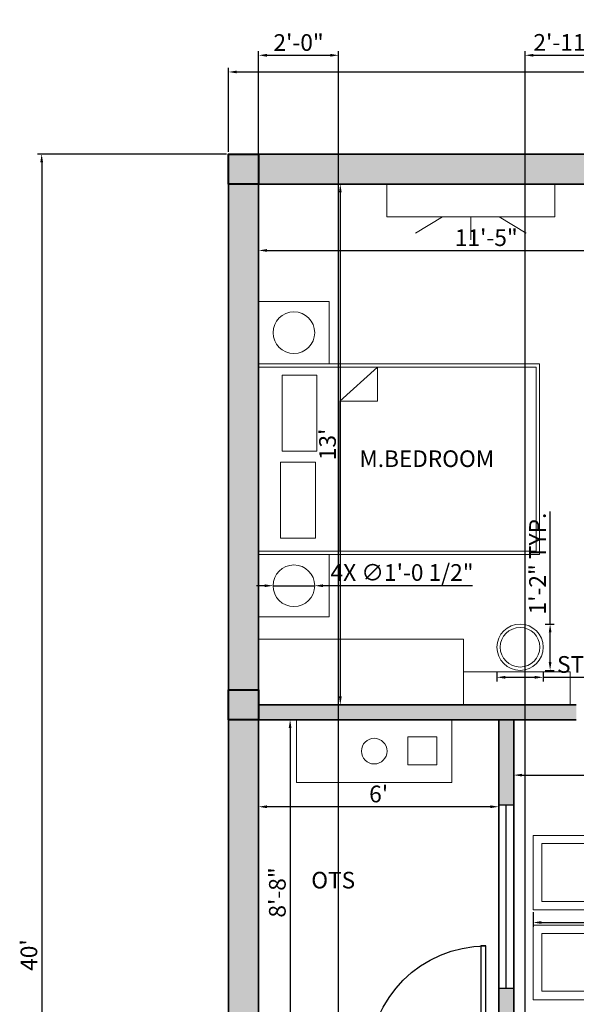
# Model space of a CAD drawing. Units: inches. Extents: x 1674 to 2231, y 1328 to 1959.
# Tile 3 of 6: x 1674 to 1841, y 1664 to 1959. Entities that reach past the tile are written whole.
import ezdxf

# ---------------------------------------------------------------- set-up
doc = ezdxf.new("R2010")
doc.units = ezdxf.units.IN
for name, color, linetype, lineweight in [('A-ANNO-DIMS', 113, 'Continuous', 18), ('A-AREA-IDEN', 113, 'Continuous', 18), ('A-COLS-PATT', 10, 'Continuous', 13), ('A-FLOR-CASE', 211, 'Continuous', 18), ('A-WALL-PATT', 140, 'Continuous', 13), ('COLUMN', 10, 'Continuous', 40), ('DOOR', 54, 'Continuous', 25), ('FUR', 211, 'Continuous', 18), ('WALL', 7, 'Continuous', 35), ('WN', 181, 'Continuous', 25)]:
    doc.layers.add(name, color=color, linetype=linetype, lineweight=lineweight)
doc.styles.get("Standard").update_dxf_attribs({"font": 'arial.ttf'})
doc.dimstyles.new('ISO-25', dxfattribs={"dimtxt": 5, "dimasz": 2.5, "dimexe": 1.25, "dimexo": 0.625, "dimtad": 1, "dimdec": 0, "dimlunit": 4, "dimtxsty": 'Standard', "dimcen": 2.5, "dimadec": 0, "dimazin": 0, "dimtfac": 1, "dimtdec": 0, "dimtmove": 0, "dimatfit": 3, "dimfxl": 1, "dimarcsym": 0})

# ---------------------------------------------------------------- blocks, each defined once
blk = doc.blocks.new('*U2')
for p, q in [((0, 0), (0, -6)), ((40, 0), (40, -6))]:
    blk.add_line(p, q)
blk.add_lwpolyline([(0, 0), (0, 40), (1.75, 40), (1.75, 0)], close=True)
blk.add_arc((0, 0), 40, 0, 90)
blk = doc.blocks.new('*D9')
at = {"layer": 'A-ANNO-DIMS', "color": 0, "lineweight": -2, "transparency": 16777216}
for p, q in [((1736.27, 1918.98), (1736.27, 1944.21)), ((2132.27, 1918.98), (2132.27, 1944.21)), ((1738.77, 1942.96), (2129.77, 1942.96))]:
    blk.add_line(p, q, dxfattribs=at)
at = {"layer": 'A-ANNO-DIMS', "color": 0, "lineweight": 100, "transparency": 16777216}
for points in [[(1738.77, 1943.37), (1738.77, 1942.54), (1736.27, 1942.96)], [(2129.77, 1943.37), (2129.77, 1942.54), (2132.27, 1942.96)]]:
    blk.add_solid(points, dxfattribs=at)
at = {"layer": 'Defpoints', "color": 0, "lineweight": 100, "transparency": 16777216}
for p in [(2132.27, 1942.96), (1736.27, 1918.36), (2132.27, 1918.36)]:
    blk.add_point(p, dxfattribs=at)
at = {"layer": 'A-ANNO-DIMS', "color": 0, "transparency": 16777216, "insert": (1934.27, 1946.13), "char_height": 5, "attachment_point": 5}
blk.add_mtext("33'", dxfattribs=at)
blk = doc.blocks.new('*D10')
at = {"layer": 'A-ANNO-DIMS', "color": 0, "lineweight": -2, "transparency": 16777216}
for p, q in [((1735.65, 1918.36), (1679.03, 1918.36)), ((1680.28, 1915.86), (1680.28, 1440.86)), ((1735.65, 1438.36), (1679.03, 1438.36))]:
    blk.add_line(p, q, dxfattribs=at)
at = {"layer": 'A-ANNO-DIMS', "color": 0, "lineweight": 100, "transparency": 16777216}
for points in [[(1679.86, 1915.86), (1680.69, 1915.86), (1680.28, 1918.36)], [(1679.86, 1440.86), (1680.69, 1440.86), (1680.28, 1438.36)]]:
    blk.add_solid(points, dxfattribs=at)
at = {"layer": 'Defpoints', "color": 0, "lineweight": 100, "transparency": 16777216}
for p in [(1736.27, 1918.36), (1680.28, 1438.36), (1736.27, 1438.36)]:
    blk.add_point(p, dxfattribs=at)
at = {"layer": 'A-ANNO-DIMS', "color": 0, "transparency": 16777216, "insert": (1677.1, 1678.36), "char_height": 5, "attachment_point": 5, "rotation": 90}
blk.add_mtext("40'", dxfattribs=at)
blk = doc.blocks.new('*D11')
at = {"layer": 'A-ANNO-DIMS', "color": 0, "lineweight": -2, "transparency": 16777216}
for p, q in [((1745.27, 1908.73), (1745.27, 1888.23)), ((1881.77, 1908.73), (1881.77, 1888.23)), ((1747.77, 1889.48), (1879.27, 1889.48))]:
    blk.add_line(p, q, dxfattribs=at)
at = {"layer": 'A-ANNO-DIMS', "color": 0, "lineweight": 100, "transparency": 16777216}
for points in [[(1747.77, 1889.9), (1747.77, 1889.07), (1745.27, 1889.48)], [(1879.27, 1889.9), (1879.27, 1889.07), (1881.77, 1889.48)]]:
    blk.add_solid(points, dxfattribs=at)
at = {"layer": 'Defpoints', "color": 0, "lineweight": 100, "transparency": 16777216}
for p in [(1745.27, 1909.36), (1881.77, 1909.36), (1881.77, 1889.48)]:
    blk.add_point(p, dxfattribs=at)
at = {"layer": 'A-ANNO-DIMS', "color": 0, "transparency": 16777216, "insert": (1813.52, 1892.66), "char_height": 5, "attachment_point": 5}
blk.add_mtext('11\'-5"', dxfattribs=at)
blk = doc.blocks.new('*D12')
at = {"layer": 'A-ANNO-DIMS', "color": 0, "lineweight": -2, "transparency": 16777216}
for p, q in [((1745.9, 1909.36), (1771.03, 1909.36)), ((1769.78, 1906.86), (1769.78, 1755.86)), ((1745.9, 1753.36), (1771.03, 1753.36))]:
    blk.add_line(p, q, dxfattribs=at)
at = {"layer": 'A-ANNO-DIMS', "color": 0, "lineweight": 100, "transparency": 16777216}
for points in [[(1769.37, 1906.86), (1770.2, 1906.86), (1769.78, 1909.36)], [(1769.37, 1755.86), (1770.2, 1755.86), (1769.78, 1753.36)]]:
    blk.add_solid(points, dxfattribs=at)
at = {"layer": 'Defpoints', "color": 0, "lineweight": 100, "transparency": 16777216}
for p in [(1745.27, 1909.36), (1745.27, 1753.36), (1769.78, 1753.36)]:
    blk.add_point(p, dxfattribs=at)
at = {"layer": 'A-ANNO-DIMS', "color": 0, "transparency": 16777216, "insert": (1766.6, 1831.36), "char_height": 5, "attachment_point": 5, "rotation": 90}
blk.add_mtext("13'", dxfattribs=at)
blk = doc.blocks.new('*D22')
at = {"layer": 'A-ANNO-DIMS', "color": 0, "lineweight": -2, "transparency": 16777216}
for p, q in [((1745.27, 1748.23), (1745.27, 1721.55)), ((1817.27, 1748.23), (1817.27, 1721.55)), ((1814.77, 1722.8), (1747.77, 1722.8))]:
    blk.add_line(p, q, dxfattribs=at)
at = {"layer": 'A-ANNO-DIMS', "color": 0, "lineweight": 100, "transparency": 16777216}
for points in [[(1747.77, 1723.22), (1747.77, 1722.39), (1745.27, 1722.8)], [(1814.77, 1723.22), (1814.77, 1722.39), (1817.27, 1722.8)]]:
    blk.add_solid(points, dxfattribs=at)
at = {"layer": 'Defpoints', "color": 0, "lineweight": 100, "transparency": 16777216}
for p in [(1745.27, 1748.86), (1817.27, 1748.86), (1745.27, 1722.8)]:
    blk.add_point(p, dxfattribs=at)
at = {"layer": 'A-ANNO-DIMS', "color": 0, "transparency": 16777216, "insert": (1781.27, 1725.98), "char_height": 5, "attachment_point": 5}
blk.add_mtext("6'", dxfattribs=at)
blk = doc.blocks.new('*D23')
at = {"layer": 'A-ANNO-DIMS', "color": 0, "lineweight": -2, "transparency": 16777216}
for p, q in [((1745.9, 1748.86), (1755.99, 1748.86)), ((1754.74, 1746.36), (1754.74, 1647.86)), ((1745.9, 1645.36), (1755.99, 1645.36))]:
    blk.add_line(p, q, dxfattribs=at)
at = {"layer": 'A-ANNO-DIMS', "color": 0, "lineweight": 100, "transparency": 16777216}
for points in [[(1754.32, 1746.36), (1755.15, 1746.36), (1754.74, 1748.86)], [(1754.32, 1647.86), (1755.15, 1647.86), (1754.74, 1645.36)]]:
    blk.add_solid(points, dxfattribs=at)
at = {"layer": 'Defpoints', "color": 0, "lineweight": 100, "transparency": 16777216}
for p in [(1745.27, 1748.86), (1745.27, 1645.36), (1754.74, 1645.36)]:
    blk.add_point(p, dxfattribs=at)
at = {"layer": 'A-ANNO-DIMS', "color": 0, "transparency": 16777216, "insert": (1751.56, 1697.11), "char_height": 5, "attachment_point": 5, "rotation": 90}
blk.add_mtext('8\'-8"', dxfattribs=at)
blk = doc.blocks.new('*D33')
at = {"layer": 'A-ANNO-DIMS', "color": 0, "lineweight": -2, "transparency": 16777216}
for p, q in [((1821.77, 1748.23), (1821.77, 1731.03)), ((2123.27, 1748.18), (2123.27, 1731.03)), ((1824.27, 1732.28), (2120.77, 1732.28))]:
    blk.add_line(p, q, dxfattribs=at)
at = {"layer": 'A-ANNO-DIMS', "color": 0, "lineweight": 100, "transparency": 16777216}
for points in [[(1824.27, 1732.69), (1824.27, 1731.86), (1821.77, 1732.28)], [(2120.77, 1732.69), (2120.77, 1731.86), (2123.27, 1732.28)]]:
    blk.add_solid(points, dxfattribs=at)
at = {"layer": 'Defpoints', "color": 0, "lineweight": 100, "transparency": 16777216}
for p in [(1821.77, 1748.86), (2123.27, 1748.81), (2123.27, 1732.28)]:
    blk.add_point(p, dxfattribs=at)
at = {"layer": 'A-ANNO-DIMS', "color": 0, "transparency": 16777216, "insert": (1972.52, 1735.45), "char_height": 5, "attachment_point": 5}
blk.add_mtext('25\'-2"', dxfattribs=at)
blk = doc.blocks.new('BED-DOUBLE-WITH-NIGHTSTANDS')
for p, q in [((35.61, 74.81), (24.38, 64.59)), ((35.61, 64.59), (35.61, 74.81)), ((24.38, 19.67), (24.38, 64.59)), ((24.38, 64.59), (35.61, 64.59))]:
    blk.add_line(p, q)
for points in [[(0, 75.81), (21.22, 75.81), (21.22, 94.48), (0, 94.48)], [(0, 19.67), (83.2, 19.67), (83.2, 74.81), (0, 74.81)], [(7.05, 49.62), (17.52, 49.62), (17.52, 72.41), (7.05, 72.41)], [(6.58, 23.6), (17.06, 23.6), (17.06, 46.39), (6.58, 46.39)], [(0, 0), (21.22, 0), (21.22, 18.67), (0, 18.67)]]:
    blk.add_lwpolyline(points, close=True)
blk.add_lwpolyline([(0, 18.67), (84.2, 18.67), (84.2, 75.81), (0, 75.81)])
for centre in [(10.61, 85.15), (10.61, 9.33)]:
    blk.add_circle(centre, 6.24)
blk = doc.blocks.new('CHAIR-DINING')
for p, q in [((21.28, 22.31), (0, 22.31)), ((0, 22.31), (0, 0)), ((21.28, 19.89), (21.28, 22.31)), ((0, 0), (21.28, 0)), ((21.28, 0), (21.28, 2.58))]:
    blk.add_line(p, q)
blk.add_lwpolyline([(25.04, 19.89), (2.65, 19.89), (2.65, 2.58), (25.04, 2.58)], close=True)
blk = doc.blocks.new('STOOL-ROUND')
for radius in [6.93, 5.93]:
    blk.add_circle((6.93, 6.93), radius)
blk = doc.blocks.new('*D40')
at = {"layer": 'A-ANNO-DIMS', "color": 0, "lineweight": -2, "transparency": 16777216}
for p, q in [((1827.55, 1691.24), (1827.55, 1686.86)), ((1852.59, 1691.24), (1852.59, 1686.86)), ((1830.05, 1688.11), (1850.09, 1688.11)), ((1852.59, 1688.11), (1936.63, 1688.11))]:
    blk.add_line(p, q, dxfattribs=at)
at = {"layer": 'A-ANNO-DIMS', "color": 0, "lineweight": 100, "transparency": 16777216}
for points in [[(1830.05, 1688.53), (1830.05, 1687.7), (1827.55, 1688.11)], [(1850.09, 1688.53), (1850.09, 1687.7), (1852.59, 1688.11)]]:
    blk.add_solid(points, dxfattribs=at)
at = {"layer": 'Defpoints', "color": 0, "lineweight": 100, "transparency": 16777216}
for p in [(1827.55, 1691.87), (1852.59, 1691.87), (1852.59, 1688.11)]:
    blk.add_point(p, dxfattribs=at)
at = {"layer": 'A-ANNO-DIMS', "color": 0, "transparency": 16777216, "insert": (1895.86, 1691.32), "char_height": 5, "attachment_point": 5}
blk.add_mtext('DINING CHAIR 2\'-1" TYP.', dxfattribs=at)
blk = doc.blocks.new('*D48')
at = {"layer": 'A-ANNO-DIMS', "color": 0, "lineweight": -2, "transparency": 16777216}
for p, q in [((1816.72, 1763.03), (1816.72, 1760.33)), ((1819.22, 1761.58), (1828.08, 1761.58)), ((1830.58, 1763.03), (1830.58, 1760.33)), ((1830.58, 1761.58), (1890.4, 1761.58))]:
    blk.add_line(p, q, dxfattribs=at)
at = {"layer": 'A-ANNO-DIMS', "color": 0, "lineweight": 100, "transparency": 16777216}
for points in [[(1819.22, 1762), (1819.22, 1761.16), (1816.72, 1761.58)], [(1828.08, 1762), (1828.08, 1761.16), (1830.58, 1761.58)]]:
    blk.add_solid(points, dxfattribs=at)
at = {"layer": 'Defpoints', "color": 0, "lineweight": 100, "transparency": 16777216}
for p in [(1816.72, 1763.66), (1830.58, 1763.66), (1830.58, 1761.58)]:
    blk.add_point(p, dxfattribs=at)
at = {"layer": 'A-ANNO-DIMS', "color": 0, "transparency": 16777216, "insert": (1861.74, 1764.79), "char_height": 5, "attachment_point": 5}
blk.add_mtext('STOOL 1\'-2" TYP.', dxfattribs=at)
blk = doc.blocks.new('*D49')
at = {"layer": 'A-ANNO-DIMS', "color": 0, "lineweight": -2, "transparency": 16777216}
for p, q in [((1832.66, 1777.53), (1832.66, 1811.28)), ((1831.21, 1777.53), (1833.91, 1777.53)), ((1832.66, 1766.16), (1832.66, 1775.03)), ((1831.21, 1763.66), (1833.91, 1763.66))]:
    blk.add_line(p, q, dxfattribs=at)
at = {"layer": 'A-ANNO-DIMS', "color": 0, "lineweight": 100, "transparency": 16777216}
for points in [[(1832.25, 1775.03), (1833.08, 1775.03), (1832.66, 1777.53)], [(1832.25, 1766.16), (1833.08, 1766.16), (1832.66, 1763.66)]]:
    blk.add_solid(points, dxfattribs=at)
at = {"layer": 'Defpoints', "color": 0, "lineweight": 100, "transparency": 16777216}
for p in [(1830.58, 1777.53), (1832.66, 1777.53), (1830.58, 1763.66)]:
    blk.add_point(p, dxfattribs=at)
at = {"layer": 'A-ANNO-DIMS', "color": 0, "transparency": 16777216, "insert": (1829.53, 1795.66), "char_height": 5, "attachment_point": 5, "rotation": 90}
blk.add_mtext('1\'-2" TYP.', dxfattribs=at)
blk = doc.blocks.new('*D54')
at = {"layer": 'A-ANNO-DIMS', "color": 0, "lineweight": -2, "transparency": 16777216}
for p, q in [((1745.27, 1575.73), (1745.27, 1949.21)), ((1747.77, 1947.96), (1766.77, 1947.96)), ((1769.27, 1575.73), (1769.27, 1949.21))]:
    blk.add_line(p, q, dxfattribs=at)
at = {"layer": 'A-ANNO-DIMS', "color": 0, "lineweight": 100, "transparency": 16777216}
for points in [[(1747.77, 1948.37), (1747.77, 1947.54), (1745.27, 1947.96)], [(1766.77, 1948.37), (1766.77, 1947.54), (1769.27, 1947.96)]]:
    blk.add_solid(points, dxfattribs=at)
at = {"layer": 'Defpoints', "color": 0, "lineweight": 100, "transparency": 16777216}
for p in [(1769.27, 1947.96), (1745.27, 1575.1), (1769.27, 1575.1)]:
    blk.add_point(p, dxfattribs=at)
at = {"layer": 'A-ANNO-DIMS', "color": 0, "transparency": 16777216, "insert": (1757.27, 1951.13), "char_height": 5, "attachment_point": 5}
blk.add_mtext('2\'-0"', dxfattribs=at)
blk = doc.blocks.new('*D56')
at = {"layer": 'A-ANNO-DIMS', "color": 0, "lineweight": -2, "transparency": 16777216}
for p, q in [((1825.14, 1600.98), (1825.14, 1949.21)), ((1827.64, 1947.96), (1858.27, 1947.96)), ((1860.77, 1600.98), (1860.77, 1949.21))]:
    blk.add_line(p, q, dxfattribs=at)
at = {"layer": 'A-ANNO-DIMS', "color": 0, "lineweight": 100, "transparency": 16777216}
for points in [[(1827.64, 1948.37), (1827.64, 1947.54), (1825.14, 1947.96)], [(1858.27, 1948.37), (1858.27, 1947.54), (1860.77, 1947.96)]]:
    blk.add_solid(points, dxfattribs=at)
at = {"layer": 'Defpoints', "color": 0, "lineweight": 100, "transparency": 16777216}
for p in [(1860.77, 1947.96), (1825.14, 1600.36), (1860.77, 1600.36)]:
    blk.add_point(p, dxfattribs=at)
at = {"layer": 'A-ANNO-DIMS', "color": 0, "transparency": 16777216, "insert": (1842.96, 1951.17), "char_height": 5, "attachment_point": 5}
blk.add_mtext('2\'-11 1/2"', dxfattribs=at)
blk = doc.blocks.new('*D59')
at = {"layer": 'A-ANNO-DIMS', "color": 0, "lineweight": -2, "transparency": 16777216}
for p, q in [((1747.14, 1789.03), (1744.64, 1789.03)), ((1749.64, 1789.03), (1762.12, 1789.03)), ((1809.43, 1789.02), (1764.62, 1789.03))]:
    blk.add_line(p, q, dxfattribs=at)
at = {"layer": 'A-ANNO-DIMS', "color": 0, "lineweight": 100, "transparency": 16777216}
for points in [[(1747.14, 1789.44), (1747.14, 1788.61), (1749.64, 1789.03)], [(1764.62, 1789.44), (1764.62, 1788.61), (1762.12, 1789.03)]]:
    blk.add_solid(points, dxfattribs=at)
at = {"layer": 'Defpoints', "color": 0, "lineweight": 100, "transparency": 16777216}
for p in [(1749.64, 1789.03), (1762.12, 1789.03)]:
    blk.add_point(p, dxfattribs=at)
at = {"layer": 'A-ANNO-DIMS', "color": 0, "transparency": 16777216, "insert": (1788.28, 1792.34), "char_height": 5, "attachment_point": 5, "rotation": 359.9983}
blk.add_mtext('4X ∅1\'-0 1/2"', dxfattribs=at)

msp = doc.modelspace()

# ---------------------------------------------------------------- hatches: boundary and pattern name
at = {"layer": 'A-COLS-PATT'}
h = msp.add_hatch(color=256, dxfattribs=at)
h.dxf.hatch_style = 1
h.paths.add_polyline_path([(1745.27, 1918.36), (1736.27, 1918.36), (1736.27, 1909.36), (1745.27, 1909.36)])
h.paths.add_polyline_path([(1886.27, 1918.36), (1877.27, 1918.36), (1877.27, 1909.36), (1886.27, 1909.36)])
h.paths.add_polyline_path([(1995.77, 1918.36), (1986.77, 1918.36), (1986.77, 1909.36), (1995.77, 1909.36)])
h.paths.add_polyline_path([(2132.27, 1918.36), (2123.27, 1918.36), (2123.27, 1909.36), (2132.27, 1909.36)])
h.paths.add_polyline_path([(1745.27, 1757.86), (1736.27, 1757.86), (1736.27, 1748.86), (1745.27, 1748.86)])
h.paths.add_polyline_path([(1886.27, 1757.86), (1877.27, 1757.86), (1877.27, 1748.86), (1886.27, 1748.86)])
h.paths.add_polyline_path([(2132.27, 1757.81), (2123.27, 1757.81), (2123.27, 1748.81), (2132.27, 1748.81)])
h.paths.add_polyline_path([(1995.77, 1757.86), (1986.77, 1757.86), (1986.77, 1748.86), (1995.77, 1748.86)])
h.paths.add_polyline_path([(2132.27, 1625.36), (2123.27, 1625.36), (2123.27, 1616.36), (2132.27, 1616.36)])
h.paths.add_polyline_path([(1995.77, 1625.36), (1986.77, 1625.36), (1986.77, 1616.36), (1995.77, 1616.36)])
h.paths.add_polyline_path([(1869.77, 1604.86), (1860.77, 1604.86), (1860.77, 1595.86), (1869.77, 1595.86)])
h.paths.add_polyline_path([(1745.27, 1609.36), (1736.27, 1609.36), (1736.27, 1600.36), (1745.27, 1600.36)])
h.paths.add_polyline_path([(1745.27, 1504.36), (1736.27, 1504.36), (1736.27, 1495.36), (1745.27, 1495.36)])
h.paths.add_polyline_path([(1870.95, 1504.36), (1861.95, 1504.36), (1861.95, 1495.36), (1870.95, 1495.36)])
h.paths.add_polyline_path([(1995.77, 1504.36), (1986.77, 1504.36), (1986.77, 1495.36), (1995.77, 1495.36)])
h.paths.add_polyline_path([(1995.77, 1447.36), (1986.77, 1447.36), (1986.77, 1438.36), (1995.77, 1438.36)])
h.paths.add_polyline_path([(2132.27, 1447.36), (2123.27, 1447.36), (2123.27, 1438.36), (2132.27, 1438.36)])
at = {"layer": 'A-WALL-PATT'}
h = msp.add_hatch(color=256, dxfattribs=at)
h.dxf.hatch_style = 1
h.paths.add_polyline_path([(1877.27, 1918.36), (1745.27, 1918.36), (1745.27, 1909.36), (1877.27, 1909.36)])
h.paths.add_polyline_path([(1986.77, 1918.36), (1886.27, 1918.36), (1886.27, 1909.36), (1986.77, 1909.36)])
h.paths.add_polyline_path([(2123.27, 1918.36), (1995.77, 1918.36), (1995.77, 1909.36), (2123.27, 1909.36)])
h.paths.add_polyline_path([(1894.11, 1861.36), (1886.27, 1861.36), (1886.27, 1865.74), (1881.77, 1865.74), (1881.77, 1808), (1881.77, 1798.89), (1884.87, 1798.89, -0.017002), (1886.27, 1798.84), (1886.27, 1852.36), (1894.11, 1852.36)])
h.paths.add_polyline_path([(1952.87, 1861.36), (1919.24, 1861.36), (1919.24, 1852.36), (1952.87, 1852.36)])
h.paths.add_polyline_path([(1991.27, 1865.74), (1986.77, 1865.74), (1986.77, 1861.36), (1976.26, 1861.36), (1976.26, 1852.36), (1986.77, 1852.36), (1986.77, 1847.49), (1986.77, 1757.86), (1991.27, 1757.86), (1991.27, 1852.36)])
h.paths.add_polyline_path([(1986.77, 1816.36), (1938.77, 1816.36), (1938.77, 1813.86), (1986.77, 1813.86)])
h.paths.add_polyline_path([(1934.27, 1819.36), (1886.27, 1819.36), (1886.27, 1816.86), (1934.27, 1816.86)])
h.paths.add_polyline_path([(1938.77, 1852.36), (1934.27, 1852.36), (1934.27, 1753.36), (1934.27, 1748.86), (1938.77, 1748.86), (1938.77, 1753.36)])
h.paths.add_polyline_path([(1934.27, 1777.36), (1915.46, 1777.36), (1886.27, 1777.36), (1886.27, 1772.86), (1934.27, 1772.86)])
h.paths.add_polyline_path([(1986.77, 1753.36), (1967.96, 1753.36), (1961.77, 1753.36, -0.017002), (1961.81, 1751.95), (1961.81, 1748.86), (1986.77, 1748.86)])
h.paths.add_polyline_path([(2000.84, 1753.36), (1995.77, 1753.36), (1995.77, 1748.86), (2000.84, 1748.86)])
h.paths.add_polyline_path([(1941.17, 1751.95), (1941.17, 1753.36), (1938.77, 1753.36), (1938.77, 1748.86), (1941.17, 1748.86)])
h.paths.add_polyline_path([(1877.27, 1753.36), (1875.49, 1753.36), (1875.49, 1748.86), (1877.27, 1748.86)])
h.paths.add_polyline_path([(1745.27, 1909.36), (1736.27, 1909.36), (1736.27, 1757.86), (1745.27, 1757.86), (1745.27, 1773.01)])
h.paths.add_polyline_path([(1778.41, 1645.36), (1745.27, 1645.36), (1745.27, 1640.86), (1778.41, 1640.86)])
h.paths.add_polyline_path([(1821.77, 1645.36), (1821.77, 1668.45), (1817.27, 1668.45), (1817.27, 1645.36), (1817.27, 1640.86), (1821.77, 1640.86)])
h.paths.add_polyline_path([(1817.27, 1645.36), (1813.39, 1645.36), (1813.39, 1640.86), (1817.27, 1640.86)])
h.paths.add_polyline_path([(1821.77, 1640.86), (1817.27, 1640.86), (1817.27, 1604.86), (1817.27, 1600.36), (1821.77, 1600.36)])
h.paths.add_polyline_path([(1825.14, 1604.86), (1821.77, 1604.86), (1821.77, 1600.36), (1825.14, 1600.36)])
h.paths.add_polyline_path([(1781.27, 1604.86), (1745.27, 1604.86), (1745.27, 1600.36), (1781.27, 1600.36)])
h = msp.add_hatch(color=256, dxfattribs=at)
h.dxf.hatch_style = 1
h.paths.add_polyline_path([(2132.27, 1909.36), (2123.27, 1909.36), (2123.27, 1757.81), (2132.27, 1757.81)], flags=17)
h.paths.add_polyline_path([(2123.27, 1753.36), (2040.84, 1753.36), (2040.84, 1748.86), (2123.27, 1748.86)], flags=17)
h.paths.add_polyline_path([(1840.51, 1753.36), (1745.27, 1753.36), (1745.27, 1748.86), (1817.27, 1748.86), (1840.51, 1748.86)], flags=17)
h.paths.add_polyline_path([(1745.27, 1748.86), (1736.27, 1748.86), (1736.27, 1609.36), (1745.27, 1609.36), (1745.27, 1640.86)], flags=17)
h.paths.add_polyline_path([(1745.27, 1600.36), (1736.27, 1600.36), (1736.27, 1504.36), (1745.27, 1504.36)], flags=17)
h.paths.add_polyline_path([(1745.27, 1495.36), (1736.27, 1495.36), (1736.27, 1447.36), (1745.27, 1447.36)], flags=17)
h.paths.add_polyline_path([(1820.35, 1504.36), (1787.69, 1504.36), (1787.69, 1495.36), (1820.35, 1495.36)], flags=17)
h.paths.add_polyline_path([(1750.58, 1504.36), (1745.27, 1504.36), (1745.27, 1495.36), (1750.58, 1495.36)], flags=17)
h.paths.add_polyline_path([(1861.95, 1504.36), (1857.47, 1504.36), (1857.47, 1495.36), (1861.95, 1495.36)], flags=17)
h.paths.add_polyline_path([(1873.66, 1504.36), (1870.95, 1504.36), (1870.95, 1495.36), (1873.66, 1495.36)], flags=17)
h.paths.add_polyline_path([(1900.85, 1501.36), (1900.85, 1504.36), (1895.88, 1504.36), (1895.88, 1495.36), (1900.85, 1495.36)], flags=17)
h.paths.add_polyline_path([(1869.77, 1595.86), (1865.27, 1595.86), (1865.27, 1504.36), (1869.77, 1504.36)], flags=17)
h.paths.add_polyline_path([(1958.26, 1504.36), (1940.74, 1504.36, -0.01877), (1940.85, 1501.36), (1940.85, 1495.36), (1958.26, 1495.36)], flags=17)
h.paths.add_polyline_path([(1995.77, 1531.51), (1986.77, 1531.51), (1986.77, 1504.36), (1995.77, 1504.36)], flags=17)
h.paths.add_polyline_path([(1986.77, 1504.36), (1980.49, 1504.36), (1980.49, 1495.36), (1986.77, 1495.36)], flags=17)
h.paths.add_polyline_path([(1995.77, 1616.36), (1986.77, 1616.36), (1986.77, 1585.02), (1995.77, 1585.02)], flags=17)
h.paths.add_polyline_path([(2000.1, 1620.86), (1995.77, 1620.86), (1995.77, 1616.36), (2000.1, 1616.36)], flags=17)
h.paths.add_polyline_path([(2053.57, 1620.86), (2040.1, 1620.86), (2040.1, 1616.36), (2053.57, 1616.36)], flags=17)
h.paths.add_polyline_path([(2123.27, 1620.86), (2109.12, 1620.86), (2109.12, 1616.36), (2123.27, 1616.36)], flags=17)
h.paths.add_polyline_path([(2132.27, 1616.36), (2123.27, 1616.36), (2123.27, 1447.36), (2132.27, 1447.36)], flags=17)
h.paths.add_polyline_path([(1986.77, 1447.36), (1870.95, 1447.36), (1870.95, 1438.36), (1986.77, 1438.36)])
h.paths.add_polyline_path([(1861.95, 1447.36), (1745.27, 1447.36), (1745.27, 1438.36), (1861.95, 1438.36)])
h.paths.add_polyline_path([(2132.27, 1918.36), (1736.27, 1918.36), (1736.27, 1504.36), (1745.27, 1504.36), (1745.27, 1600.36), (1745.27, 1909.36), (2123.27, 1909.36), (2123.27, 1447.36), (2132.27, 1447.36)])
h = msp.add_hatch(color=256, dxfattribs=at)
h.dxf.hatch_style = 1
h.paths.add_polyline_path([(1886.27, 1777.36), (1886.27, 1778.24), (1884.87, 1778.24), (1881.77, 1778.24), (1881.77, 1757.86), (1886.27, 1757.86)], flags=17)
h.paths.add_polyline_path([(2132.27, 1918.36), (1736.27, 1918.36), (1736.27, 1757.86), (1745.27, 1757.86), (1745.27, 1773.01), (1745.27, 1909.36), (2123.27, 1909.36), (2123.27, 1757.81), (2132.27, 1757.81)])
h = msp.add_hatch(color=256, dxfattribs=at)
h.dxf.hatch_style = 1
h.paths.add_polyline_path([(1745.27, 1600.36), (1736.27, 1600.36), (1736.27, 1504.36), (1745.27, 1504.36)])
h.paths.add_polyline_path([(1745.27, 1748.86), (1736.27, 1748.86), (1736.27, 1609.36), (1745.27, 1609.36), (1745.27, 1640.86)])
h.paths.add_polyline_path([(1821.77, 1748.86), (1817.27, 1748.86), (1817.27, 1723.23), (1821.77, 1723.23)])

# ---------------------------------------------------------------- linework, layer by layer
at = {"layer": 'A-FLOR-CASE'}
for points in [[(1745.27, 1753.36), (1806.75, 1753.36), (1806.75, 1773.01), (1745.27, 1773.01)], [(1806.75, 1763.18), (1838.68, 1763.18), (1838.68, 1753.36), (1806.75, 1753.36)], [(1756.7, 1748.86), (1803.2, 1748.86), (1803.2, 1730.07), (1756.7, 1730.07)], [(1798.71, 1743.79), (1789.98, 1743.79), (1789.98, 1735.36), (1798.71, 1735.36)]]:
    msp.add_lwpolyline(points, close=True, dxfattribs=at)
msp.add_circle((1779.95, 1739.46), 3.84, dxfattribs=at)
at = {"layer": 'COLUMN'}
for points in [[(1736.27, 1918.36), (1745.27, 1918.36), (1745.27, 1909.36), (1736.27, 1909.36)], [(1736.27, 1757.86), (1745.27, 1757.86), (1745.27, 1748.86), (1736.27, 1748.86)]]:
    msp.add_lwpolyline(points, close=True, dxfattribs=at)
at = {"layer": 'FUR'}
for p, q in [((1800.42, 1899.54), (1792.31, 1894.64)), ((1808.89, 1899.54), (1808.89, 1892.66)), ((1817.37, 1899.54), (1825.48, 1894.64))]:
    msp.add_line(p, q, dxfattribs=at)
msp.add_lwpolyline([(1783.71, 1909.36), (1834.08, 1909.36), (1834.08, 1899.54), (1783.71, 1899.54)], close=True, dxfattribs=at)
at = {"layer": 'WALL'}
for p, q in [((1736.27, 1918.36), (2132.27, 1918.36)), ((1736.27, 1438.36), (1736.27, 1918.36)), ((1745.27, 1909.36), (1881.77, 1909.36)), ((1840.51, 1753.36), (1745.27, 1753.36)), ((1745.27, 1748.86), (1817.27, 1748.86)), ((1840.51, 1748.86), (1745.27, 1748.86)), ((1817.27, 1748.86), (1817.27, 1645.36)), ((1821.77, 1748.86), (1821.77, 1640.86))]:
    msp.add_line(p, q, dxfattribs=at)
for points in [[(1995.77, 1438.36), (1736.27, 1438.36), (1736.27, 1918.36), (2132.27, 1918.36), (2132.27, 1438.36), (2123.27, 1438.36)], [(1995.77, 1447.36), (1745.27, 1447.36), (1745.27, 1909.36), (2123.27, 1909.36), (2123.27, 1447.36)]]:
    msp.add_lwpolyline(points, dxfattribs=at)
at = {"layer": 'WN'}
msp.add_line((1819.52, 1668.45), (1819.52, 1723.23), dxfattribs=at)
msp.add_lwpolyline([(1817.27, 1668.45), (1821.77, 1668.45), (1821.77, 1723.23), (1817.27, 1723.23)], close=True, dxfattribs=at)

# ---------------------------------------------------------------- block references
at = {"layer": 'DOOR', "xscale": -0.8744829560094038, "yscale": 0.8744829560094038, "zscale": 0.8744829560094038}
msp.add_blockref('*U2', (1813.39, 1646.1), dxfattribs=at)
at = {"layer": 'FUR'}
for name, p in [('BED-DOUBLE-WITH-NIGHTSTANDS', (1745.27, 1779.69)), ('STOOL-ROUND', (1816.72, 1763.66)), ('CHAIR-DINING', (1827.55, 1691.87)), ('CHAIR-DINING', (1827.55, 1664.98))]:
    msp.add_blockref(name, p, dxfattribs=at)

# ---------------------------------------------------------------- texts
at = {"layer": 'A-AREA-IDEN', "char_height": 4.973, "attachment_point": 1}
for s, insert in [('M.BEDROOM', (1775.5, 1829.57)), ('OTS', (1761.08, 1703.29))]:
    msp.add_mtext_dynamic_manual_height_columns(s, width=89.7127, gutter_width=24.87, heights=[0], dxfattribs=dict(at, insert=insert))

# ---------------------------------------------------------------- dimensions: what is measured, and where the dimension line sits
at = {"layer": 'A-ANNO-DIMS'}
for base, p1, p2, override, picture, middle in [((1860.77, 1947.96), (1825.14, 1600.36), (1860.77, 1600.36), {"dimdec": 1, "dimlfac": 1, "dimrnd": 0, "dimzin": 1, "dimdsep": 46, "dimlunit": 4, "dimfrac": 2}, '*D56', (1842.96, 1951.17)), ((1769.27, 1947.96), (1745.27, 1575.1), (1769.27, 1575.1), {"dimdec": 1, "dimlfac": 1, "dimrnd": 0, "dimzin": 1, "dimdsep": 46, "dimlunit": 4, "dimfrac": 2}, '*D54', (1757.27, 1951.13)), ((2132.27, 1942.96), (1736.27, 1918.36), (2132.27, 1918.36), {"dimclrd": 0, "dimclre": 0, "dimclrt": 0}, '*D9', (1934.27, 1946.13)), ((1881.77109151, 1889.48404083), (1745.27109151, 1909.35548105), (1881.77109151, 1909.35548105), {"dimclrd": 0, "dimclre": 0, "dimclrt": 0}, '*D11', (1813.52109151, 1892.66190577)), ((1745.27, 1722.8), (1817.27, 1748.86), (1745.27, 1748.86), {"dimclrd": 0, "dimclre": 0, "dimclrt": 0}, '*D22', (1781.27, 1725.98)), ((2123.27109151, 1732.2761534), (1821.77109151, 1748.85548105), (2123.27109151, 1748.80863988), {"dimclrd": 0, "dimclre": 0, "dimclrt": 0}, '*D33', (1972.52109151, 1735.45401834))]:
    dim = msp.add_linear_dim(base=base, p1=p1, p2=p2, dimstyle='ISO-25', override=override, dxfattribs=at)
    dim.commit()
    dim.dimension.update_dxf_attribs({"geometry": picture, "text_midpoint": middle})
for base, p1, p2, picture, middle in [((1680.28, 1438.36), (1736.27, 1918.36), (1736.27, 1438.36), '*D10', (1677.1, 1678.36)), ((1769.78, 1753.36), (1745.27, 1909.36), (1745.27, 1753.36), '*D12', (1766.6, 1831.36)), ((1754.73763243, 1645.35548105), (1745.27109151, 1748.85548105), (1745.27109151, 1645.35548105), '*D23', (1751.55976749, 1697.10548105))]:
    dim = msp.add_linear_dim(base=base, p1=p1, p2=p2, angle=90, dimstyle='ISO-25', override={"dimclrd": 0, "dimclre": 0, "dimclrt": 0}, dxfattribs=at)
    dim.commit()
    dim.dimension.update_dxf_attribs({"geometry": picture, "text_midpoint": middle})
dim = msp.add_linear_dim(base=(1832.66, 1777.53), p1=(1830.58, 1763.66), p2=(1830.58, 1777.53), angle=90, text='<> TYP.', dimstyle='ISO-25', override={"dimdec": 1, "dimlfac": 1, "dimrnd": 0, "dimzin": 1, "dimdsep": 46, "dimlunit": 4, "dimfrac": 2}, dxfattribs=at)
dim.commit()
dim.dimension.update_dxf_attribs({"geometry": '*D49', "text_midpoint": (1829.53, 1795.66)})
dim = msp.add_diameter_dim_2p(p1=(1749.64, 1789.03), p2=(1762.12, 1789.03), text='4X <>', dimstyle='ISO-25', override={"dimdec": 1, "dimlfac": 1, "dimrnd": 0, "dimzin": 1, "dimdsep": 46, "dimlunit": 4, "dimfrac": 2}, dxfattribs=at)
dim.commit()
dim.dimension.update_dxf_attribs({"geometry": '*D59', "text_midpoint": (1788.28, 1789.03), "dimtype": 163})
for base, p1, p2, text, picture, middle in [((1830.58, 1761.58), (1816.72, 1763.66), (1830.58, 1763.66), 'STOOL <> TYP.', '*D48', (1861.74, 1764.79)), ((1852.59, 1688.11), (1827.55, 1691.87), (1852.59, 1691.87), 'DINING CHAIR <> TYP.', '*D40', (1895.86, 1691.32))]:
    dim = msp.add_linear_dim(base=base, p1=p1, p2=p2, text=text, dimstyle='ISO-25', override={"dimdec": 1, "dimlfac": 1, "dimrnd": 0, "dimzin": 1, "dimdsep": 46, "dimlunit": 4, "dimfrac": 2}, dxfattribs=at)
    dim.commit()
    dim.dimension.update_dxf_attribs({"geometry": picture, "text_midpoint": middle})

doc.saveas('drawing.dxf')
